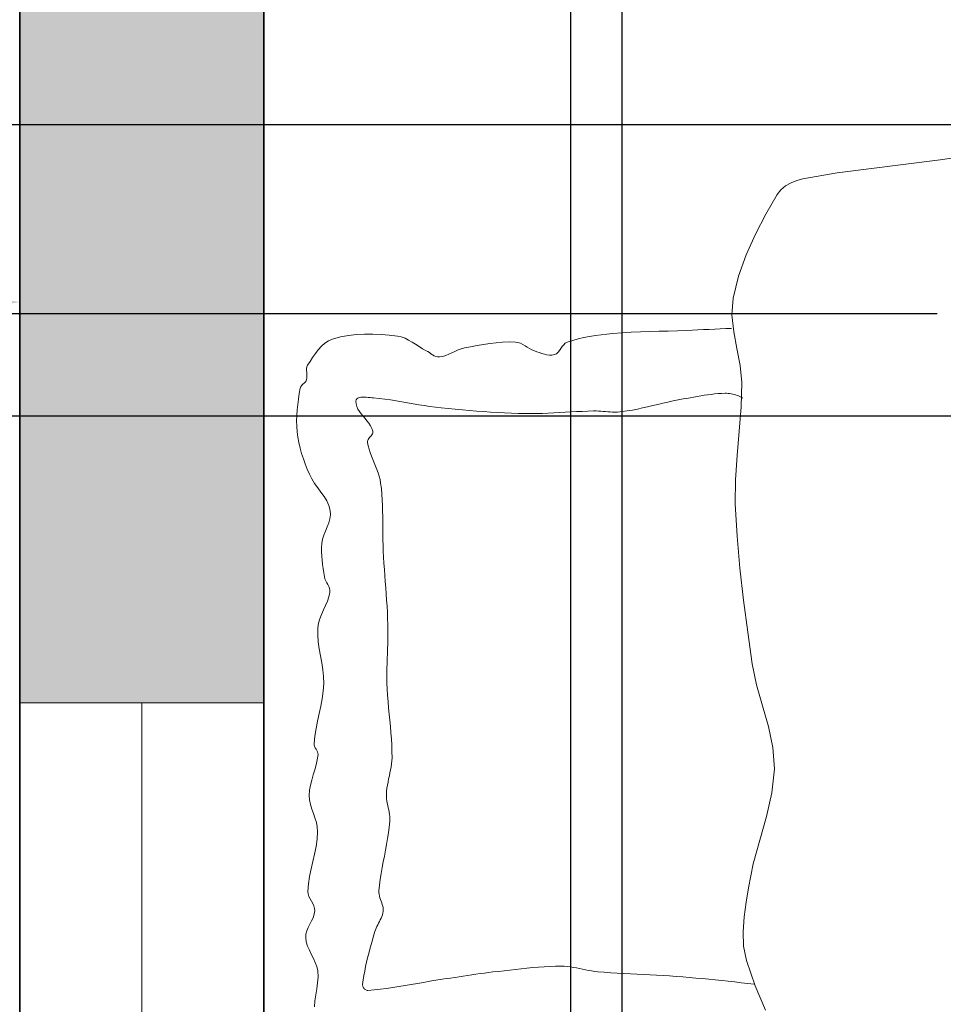
# Model space of a CAD drawing. Units: inches. Extents: x 2656 to 9931, y 1941 to 3068.
# Tile 10 of 46: x 2743 to 2777, y 2533 to 2569. Entities that reach past the tile are written whole.
import ezdxf

# ---------------------------------------------------------------- set-up
doc = ezdxf.new("R2010")
doc.units = ezdxf.units.IN
for name, color, linetype, lineweight in [('A-ANNO-DIMS', 2, 'Continuous', 18), ('A-FURN', 8, 'Continuous', 13), ('A-GLAZ', 4, 'Continuous', 18), ('A-WALL', 7, 'Continuous', 35), ('A-WALL-PATT', 251, 'Continuous', 13)]:
    doc.layers.add(name, color=color, linetype=linetype, lineweight=lineweight)
doc.styles.get("Standard").update_dxf_attribs({"font": 'arial.ttf'})
doc.dimstyles.new('ISO-25', dxfattribs={"dimtxt": 6, "dimasz": 2.5, "dimexe": 1.25, "dimexo": 0.625, "dimtad": 1, "dimdec": 0, "dimlunit": 3, "dimtxsty": 'Standard', "dimcen": 2.5, "dimadec": 0, "dimazin": 0, "dimtfac": 1, "dimtdec": 0, "dimtmove": 0, "dimatfit": 3, "dimfxl": 1, "dimarcsym": 0})

# ---------------------------------------------------------------- blocks, each defined once
blk = doc.blocks.new('*D1')
at = {"layer": 'A-ANNO-DIMS', "color": 0, "lineweight": -2, "transparency": 16777216}
for p, q in [((2728.157, 2559.424), (2728.157, 2560.049)), ((2743.157, 2559.424), (2743.157, 2560.049)), ((2730.657, 2558.799), (2740.657, 2558.799))]:
    blk.add_line(p, q, dxfattribs=at)
at = {"layer": 'A-ANNO-DIMS', "color": 0, "transparency": 16777216}
for points in [[(2730.657, 2559.216), (2730.657, 2558.383), (2728.157, 2558.799)], [(2740.657, 2559.216), (2740.657, 2558.383), (2743.157, 2558.799)]]:
    blk.add_solid(points, dxfattribs=at)
at = {"layer": 'Defpoints', "color": 0, "transparency": 16777216}
for p in [(2728.157, 2558.799), (2743.157, 2558.799), (2743.157, 2558.799)]:
    blk.add_point(p, dxfattribs=at)
at = {"layer": 'A-ANNO-DIMS', "color": 0, "transparency": 16777216, "insert": (2735.657, 2562.49), "char_height": 6, "attachment_point": 5}
blk.add_mtext('1\'3"', dxfattribs=at)
blk = doc.blocks.new('BED-DOUBLE')
for p, q in [((24.929, 61.432), (23.668, 61.237)), ((22.401, 61.078), (21.133, 60.928)), ((23.668, 61.237), (22.401, 61.078)), ((19.868, 60.758), (18.612, 60.54)), ((21.133, 60.928), (19.868, 60.758)), ((17.974, 60.285), (17.799, 60.142)), ((18.176, 60.399), (17.974, 60.285)), ((18.392, 60.483), (18.176, 60.399)), ((18.612, 60.54), (18.392, 60.483)), ((17.664, 59.967), (17.251, 59.242)), ((17.799, 60.142), (17.664, 59.967)), ((17.251, 59.242), (16.864, 58.499)), ((16.864, 58.499), (16.52, 57.736)), ((16.52, 57.736), (16.239, 56.953)), ((16.239, 56.953), (16.039, 56.149)), ((16.039, 56.149), (15.997, 55.53)), ((15.997, 55.53), (16.064, 54.908)), ((2.165, 54.807), (1.867, 54.773)), ((2.466, 54.823), (2.165, 54.807)), ((2.769, 54.822), (2.466, 54.823)), ((3.071, 54.807), (2.769, 54.822)), ((3.373, 54.782), (3.071, 54.807)), ((11.392, 54.817), (11.179, 54.792)), ((11.605, 54.838), (11.392, 54.817)), ((11.945, 54.867), (11.605, 54.838)), ((12.285, 54.889), (11.945, 54.867)), ((12.626, 54.904), (12.285, 54.889)), ((12.968, 54.916), (12.626, 54.904)), ((13.309, 54.925), (12.968, 54.916)), ((13.651, 54.933), (13.309, 54.925)), ((13.992, 54.943), (13.651, 54.933)), ((14.333, 54.956), (13.992, 54.943)), ((14.539, 54.965), (14.333, 54.956)), ((14.745, 54.974), (14.539, 54.965)), ((14.951, 54.984), (14.745, 54.974)), ((15.157, 54.993), (14.951, 54.984)), ((15.363, 55.002), (15.157, 54.993)), ((15.569, 55.012), (15.363, 55.002)), ((15.775, 55.021), (15.569, 55.012)), ((15.98, 55.031), (15.775, 55.021)), ((16.064, 54.908), (16.183, 54.283)), ((0.997, 54.482), (0.871, 54.371)), ((1.134, 54.573), (0.997, 54.482)), ((1.286, 54.638), (1.134, 54.573)), ((1.573, 54.718), (1.286, 54.638)), ((1.867, 54.773), (1.573, 54.718)), ((3.671, 54.748), (3.373, 54.782)), ((3.815, 54.718), (3.671, 54.748)), ((3.953, 54.668), (3.815, 54.718)), ((4.086, 54.602), (3.953, 54.668)), ((4.216, 54.525), (4.086, 54.602)), ((4.344, 54.443), (4.216, 54.525)), ((4.471, 54.359), (4.344, 54.443)), ((6.84, 54.439), (6.605, 54.399)), ((7.076, 54.474), (6.84, 54.439)), ((7.312, 54.503), (7.076, 54.474)), ((7.548, 54.522), (7.312, 54.503)), ((7.785, 54.531), (7.548, 54.522)), ((8.022, 54.528), (7.785, 54.531)), ((8.115, 54.514), (8.022, 54.528)), ((8.204, 54.483), (8.115, 54.514)), ((8.29, 54.44), (8.204, 54.483)), ((8.374, 54.39), (8.29, 54.44)), ((9.858, 54.484), (9.799, 54.428)), ((9.929, 54.522), (9.858, 54.484)), ((10.131, 54.589), (9.929, 54.522)), ((10.337, 54.645), (10.131, 54.589)), ((10.545, 54.692), (10.337, 54.645)), ((10.755, 54.732), (10.545, 54.692)), ((10.967, 54.765), (10.755, 54.732)), ((11.179, 54.792), (10.967, 54.765)), ((0.65, 54.106), (0.55, 53.961)), ((0.756, 54.244), (0.65, 54.106)), ((0.871, 54.371), (0.756, 54.244)), ((4.6, 54.279), (4.471, 54.359)), ((4.732, 54.207), (4.6, 54.279)), ((4.791, 54.174), (4.732, 54.207)), ((4.85, 54.136), (4.791, 54.174)), ((4.909, 54.096), (4.85, 54.136)), ((4.968, 54.058), (4.909, 54.096)), ((5.568, 54.077), (5.454, 54.031)), ((5.68, 54.13), (5.568, 54.077)), ((5.792, 54.184), (5.68, 54.13)), ((5.905, 54.235), (5.792, 54.184)), ((6.02, 54.279), (5.905, 54.235)), ((6.138, 54.31), (6.02, 54.279)), ((6.371, 54.355), (6.138, 54.31)), ((6.605, 54.399), (6.371, 54.355)), ((8.458, 54.336), (8.374, 54.39)), ((8.542, 54.284), (8.458, 54.336)), ((8.628, 54.237), (8.542, 54.284)), ((8.717, 54.201), (8.628, 54.237)), ((8.808, 54.17), (8.717, 54.201)), ((8.9, 54.138), (8.808, 54.17)), ((8.993, 54.107), (8.9, 54.138)), ((9.087, 54.08), (8.993, 54.107)), ((9.181, 54.059), (9.087, 54.08)), ((9.532, 54.097), (9.459, 54.064)), ((9.593, 54.149), (9.532, 54.097)), ((9.647, 54.214), (9.593, 54.149)), ((9.696, 54.287), (9.647, 54.214)), ((9.746, 54.36), (9.696, 54.287)), ((9.799, 54.428), (9.746, 54.36)), ((16.183, 54.283), (16.3, 53.657)), ((0.456, 53.815), (0.365, 53.671)), ((0.55, 53.961), (0.456, 53.815)), ((5.028, 54.024), (4.968, 54.058)), ((5.089, 53.997), (5.028, 54.024)), ((5.153, 53.981), (5.089, 53.997)), ((5.218, 53.978), (5.153, 53.981)), ((5.338, 53.997), (5.218, 53.978)), ((5.454, 54.031), (5.338, 53.997)), ((9.274, 54.048), (9.181, 54.059)), ((9.367, 54.049), (9.274, 54.048)), ((9.459, 54.064), (9.367, 54.049)), ((0.326, 53.548), (0.324, 53.481)), ((0.324, 53.481), (0.33, 53.412)), ((0.337, 53.612), (0.326, 53.548)), ((0.33, 53.412), (0.337, 53.342)), ((0.365, 53.671), (0.337, 53.612)), ((16.3, 53.657), (16.356, 53.03)), ((0.241, 53.017), (0.203, 52.982)), ((0.276, 53.054), (0.241, 53.017)), ((0.306, 53.094), (0.276, 53.054)), ((0.326, 53.138), (0.306, 53.094)), ((0.339, 53.203), (0.326, 53.138)), ((0.337, 53.342), (0.341, 53.272)), ((0.341, 53.272), (0.339, 53.203)), ((16.356, 53.03), (16.332, 52.135)), ((0.058, 52.625), (0.027, 52.426)), ((0.093, 52.823), (0.058, 52.625)), ((0.108, 52.868), (0.093, 52.823)), ((0.134, 52.909), (0.108, 52.868)), ((0.167, 52.946), (0.134, 52.909)), ((0.203, 52.982), (0.167, 52.946)), ((15.359, 52.614), (15.488, 52.625)), ((15.488, 52.625), (15.617, 52.633)), ((15.617, 52.633), (15.747, 52.637)), ((15.747, 52.637), (15.802, 52.637)), ((15.802, 52.637), (15.858, 52.634)), ((15.858, 52.634), (15.913, 52.628)), ((15.913, 52.628), (15.969, 52.619)), ((0.027, 52.426), (0, 52.226)), ((2.14, 52.349), (2.15, 52.398)), ((2.149, 52.246), (2.14, 52.349)), ((2.15, 52.398), (2.175, 52.435)), ((2.175, 52.435), (2.213, 52.463)), ((2.213, 52.463), (2.262, 52.481)), ((2.262, 52.481), (2.32, 52.492)), ((2.32, 52.492), (2.384, 52.497)), ((2.384, 52.497), (2.453, 52.497)), ((2.453, 52.497), (2.525, 52.494)), ((2.525, 52.494), (2.597, 52.487)), ((2.597, 52.487), (2.666, 52.48)), ((2.666, 52.48), (2.731, 52.473)), ((2.731, 52.473), (2.79, 52.468)), ((2.79, 52.468), (3, 52.448)), ((3, 52.448), (3.209, 52.423)), ((3.209, 52.423), (3.417, 52.394)), ((3.417, 52.394), (3.625, 52.362)), ((3.625, 52.362), (3.833, 52.327)), ((3.833, 52.327), (4.041, 52.291)), ((4.041, 52.291), (4.248, 52.254)), ((13.267, 52.226), (13.454, 52.269)), ((13.454, 52.269), (13.641, 52.312)), ((13.641, 52.312), (13.829, 52.354)), ((13.829, 52.354), (14.017, 52.392)), ((14.017, 52.392), (14.206, 52.428)), ((14.206, 52.428), (14.333, 52.451)), ((14.333, 52.451), (14.461, 52.474)), ((14.461, 52.474), (14.589, 52.498)), ((14.589, 52.498), (14.717, 52.521)), ((14.717, 52.521), (14.845, 52.543)), ((14.845, 52.543), (14.973, 52.563)), ((14.973, 52.563), (15.102, 52.582)), ((15.102, 52.582), (15.23, 52.599)), ((15.23, 52.599), (15.359, 52.614)), ((15.969, 52.619), (16.024, 52.608)), ((16.024, 52.608), (16.079, 52.595)), ((16.079, 52.595), (16.133, 52.579)), ((16.133, 52.579), (16.186, 52.561)), ((16.186, 52.561), (16.238, 52.54)), ((16.238, 52.54), (16.289, 52.517)), ((16.289, 52.517), (16.338, 52.491)), ((16.338, 52.491), (16.386, 52.464)), ((-0.022, 52.025), (-0.036, 51.824)), ((0, 52.226), (-0.022, 52.025)), ((2.176, 52.149), (2.149, 52.246)), ((2.219, 52.056), (2.176, 52.149)), ((2.274, 51.966), (2.219, 52.056)), ((2.338, 51.878), (2.274, 51.966)), ((4.248, 52.254), (4.456, 52.218)), ((4.456, 52.218), (4.664, 52.184)), ((4.664, 52.184), (4.872, 52.152)), ((4.872, 52.152), (5.081, 52.123)), ((5.081, 52.123), (5.29, 52.099)), ((5.29, 52.099), (5.548, 52.073)), ((5.548, 52.073), (5.806, 52.048)), ((5.806, 52.048), (6.065, 52.025)), ((6.065, 52.025), (6.323, 52.003)), ((6.323, 52.003), (6.582, 51.982)), ((6.582, 51.982), (6.841, 51.963)), ((6.841, 51.963), (7.1, 51.946)), ((7.1, 51.946), (7.359, 51.931)), ((7.359, 51.931), (7.618, 51.918)), ((7.618, 51.918), (7.877, 51.907)), ((7.877, 51.907), (8.136, 51.898)), ((8.136, 51.898), (8.396, 51.891)), ((8.813, 51.891), (9.022, 51.897)), ((9.022, 51.897), (9.231, 51.905)), ((9.231, 51.905), (9.44, 51.915)), ((9.44, 51.915), (9.648, 51.927)), ((9.648, 51.927), (9.857, 51.939)), ((9.857, 51.939), (10.066, 51.951)), ((10.066, 51.951), (10.275, 51.963)), ((10.275, 51.963), (10.483, 51.973)), ((10.483, 51.973), (10.692, 51.981)), ((10.692, 51.981), (10.901, 51.987)), ((10.901, 51.987), (10.989, 51.987)), ((10.989, 51.987), (11.076, 51.984)), ((11.076, 51.984), (11.164, 51.979)), ((11.164, 51.979), (11.251, 51.973)), ((11.251, 51.973), (11.339, 51.966)), ((11.339, 51.966), (11.427, 51.959)), ((11.427, 51.959), (11.514, 51.953)), ((11.514, 51.953), (11.601, 51.948)), ((11.601, 51.948), (11.689, 51.946)), ((11.689, 51.946), (11.776, 51.947)), ((11.776, 51.947), (11.863, 51.952)), ((11.863, 51.952), (11.95, 51.961)), ((11.95, 51.961), (12.14, 51.989)), ((12.14, 51.989), (12.329, 52.021)), ((12.329, 52.021), (12.517, 52.058)), ((12.517, 52.058), (12.705, 52.097)), ((12.705, 52.097), (12.892, 52.139)), ((12.892, 52.139), (13.08, 52.182)), ((13.08, 52.182), (13.267, 52.226)), ((16.332, 52.135), (16.264, 51.241)), ((-0.036, 51.824), (-0.042, 51.623)), ((-0.042, 51.623), (-0.038, 51.422)), ((2.408, 51.792), (2.338, 51.878)), ((2.481, 51.706), (2.408, 51.792)), ((2.552, 51.62), (2.481, 51.706)), ((2.62, 51.532), (2.552, 51.62)), ((8.396, 51.891), (8.604, 51.889)), ((8.604, 51.889), (8.813, 51.891)), ((-0.038, 51.422), (-0.022, 51.223)), ((-0.022, 51.223), (0.005, 51.02)), ((2.681, 51.441), (2.62, 51.532)), ((2.731, 51.346), (2.681, 51.441)), ((2.768, 51.248), (2.731, 51.346)), ((2.752, 51.141), (2.767, 51.176)), ((2.767, 51.176), (2.773, 51.211)), ((2.773, 51.211), (2.768, 51.248)), ((16.264, 51.241), (16.184, 50.347)), ((0.005, 51.02), (0.042, 50.82)), ((0.042, 50.82), (0.09, 50.62)), ((2.572, 50.868), (2.582, 50.904)), ((2.572, 50.83), (2.572, 50.868)), ((2.597, 50.702), (2.572, 50.83)), ((2.582, 50.904), (2.599, 50.939)), ((2.599, 50.939), (2.622, 50.973)), ((2.622, 50.973), (2.649, 51.007)), ((2.649, 51.007), (2.678, 51.041)), ((2.678, 51.041), (2.706, 51.074)), ((2.706, 51.074), (2.731, 51.108)), ((2.731, 51.108), (2.752, 51.141)), ((0.09, 50.62), (0.145, 50.423)), ((2.63, 50.575), (2.597, 50.702)), ((2.67, 50.45), (2.63, 50.575)), ((2.715, 50.326), (2.67, 50.45)), ((0.145, 50.423), (0.208, 50.227)), ((0.208, 50.227), (0.277, 50.034)), ((2.764, 50.203), (2.715, 50.326)), ((2.815, 50.081), (2.764, 50.203)), ((2.865, 49.958), (2.815, 50.081)), ((16.184, 50.347), (16.125, 49.453)), ((0.277, 50.034), (0.35, 49.842)), ((0.35, 49.842), (0.428, 49.653)), ((2.914, 49.835), (2.865, 49.958)), ((2.959, 49.711), (2.914, 49.835)), ((0.428, 49.653), (0.515, 49.48)), ((0.515, 49.48), (0.62, 49.315)), ((2.999, 49.586), (2.959, 49.711)), ((3.032, 49.459), (2.999, 49.586)), ((3.055, 49.331), (3.032, 49.459)), ((16.125, 49.453), (16.121, 48.558)), ((0.62, 49.315), (0.736, 49.155)), ((0.736, 49.155), (0.854, 48.996)), ((0.854, 48.996), (0.968, 48.836)), ((3.082, 49.123), (3.055, 49.331)), ((3.101, 48.916), (3.082, 49.123)), ((0.968, 48.836), (1.068, 48.671)), ((1.068, 48.671), (1.148, 48.498)), ((3.115, 48.707), (3.101, 48.916)), ((3.124, 48.499), (3.115, 48.707)), ((1.148, 48.498), (1.199, 48.315)), ((1.199, 48.315), (1.208, 48.162)), ((3.129, 48.29), (3.124, 48.499)), ((3.132, 48.081), (3.129, 48.29)), ((16.121, 48.558), (16.187, 47.374)), ((1.186, 48.011), (1.142, 47.861)), ((1.208, 48.162), (1.186, 48.011)), ((3.133, 47.871), (3.132, 48.081)), ((1.02, 47.562), (0.96, 47.411)), ((1.083, 47.712), (1.02, 47.562)), ((1.142, 47.861), (1.083, 47.712)), ((3.134, 47.662), (3.133, 47.871)), ((3.135, 47.452), (3.134, 47.662)), ((0.912, 47.259), (0.885, 47.105)), ((0.96, 47.411), (0.912, 47.259)), ((3.137, 47.243), (3.135, 47.452)), ((3.142, 47.034), (3.137, 47.243)), ((16.187, 47.374), (16.29, 46.193)), ((0.885, 47.105), (0.876, 46.95)), ((0.876, 46.95), (0.876, 46.796)), ((3.151, 46.825), (3.142, 47.034)), ((3.163, 46.599), (3.151, 46.825)), ((0.876, 46.796), (0.882, 46.641)), ((0.882, 46.641), (0.895, 46.486)), ((0.895, 46.486), (0.913, 46.331)), ((3.178, 46.373), (3.163, 46.599)), ((0.913, 46.331), (0.935, 46.177)), ((0.935, 46.177), (0.959, 46.023)), ((3.193, 46.147), (3.178, 46.373)), ((3.209, 45.922), (3.193, 46.147)), ((16.29, 46.193), (16.422, 45.014)), ((0.959, 46.023), (0.984, 45.87)), ((0.984, 45.87), (1.003, 45.798)), ((1.003, 45.798), (1.033, 45.727)), ((1.033, 45.727), (1.069, 45.658)), ((3.226, 45.696), (3.209, 45.922)), ((1.069, 45.658), (1.107, 45.59)), ((1.107, 45.59), (1.143, 45.521)), ((1.143, 45.521), (1.17, 45.452)), ((1.17, 45.452), (1.187, 45.381)), ((1.187, 45.381), (1.187, 45.308)), ((3.243, 45.47), (3.226, 45.696)), ((3.259, 45.245), (3.243, 45.47)), ((1.151, 45.139), (1.095, 44.974)), ((1.187, 45.308), (1.151, 45.139)), ((3.275, 45.019), (3.259, 45.245)), ((3.289, 44.793), (3.275, 45.019)), ((16.422, 45.014), (16.577, 43.838)), ((0.951, 44.651), (0.877, 44.491)), ((1.026, 44.812), (0.951, 44.651)), ((1.095, 44.974), (1.026, 44.812)), ((3.302, 44.567), (3.289, 44.793)), ((0.812, 44.328), (0.763, 44.162)), ((0.877, 44.491), (0.812, 44.328)), ((3.312, 44.341), (3.302, 44.567)), ((3.32, 44.115), (3.312, 44.341)), ((0.738, 43.992), (0.735, 43.734)), ((0.763, 44.162), (0.738, 43.992)), ((3.323, 43.936), (3.32, 44.115)), ((3.323, 43.757), (3.323, 43.936)), ((0.735, 43.734), (0.756, 43.477)), ((3.315, 43.399), (3.32, 43.578)), ((3.32, 43.578), (3.323, 43.757)), ((16.577, 43.838), (16.745, 42.664)), ((0.756, 43.477), (0.793, 43.221)), ((0.793, 43.221), (0.839, 42.964)), ((3.302, 43.041), (3.309, 43.22)), ((3.309, 43.22), (3.315, 43.399)), ((0.839, 42.964), (0.887, 42.708)), ((3.289, 42.683), (3.295, 42.862)), ((3.295, 42.862), (3.302, 43.041)), ((0.887, 42.708), (0.928, 42.451)), ((3.282, 42.325), (3.285, 42.504)), ((3.285, 42.504), (3.289, 42.683)), ((16.745, 42.664), (16.906, 41.889)), ((0.928, 42.451), (0.954, 42.194)), ((0.954, 42.194), (0.959, 41.936)), ((3.283, 42.146), (3.282, 42.325)), ((3.286, 41.967), (3.283, 42.146)), ((0.959, 41.936), (0.94, 41.658)), ((3.296, 41.737), (3.286, 41.967)), ((3.311, 41.506), (3.296, 41.737)), ((16.906, 41.889), (17.122, 41.121)), ((0.902, 41.381), (0.851, 41.106)), ((0.94, 41.658), (0.902, 41.381)), ((3.328, 41.276), (3.311, 41.506)), ((0.851, 41.106), (0.794, 40.832)), ((3.349, 41.046), (3.328, 41.276)), ((3.371, 40.816), (3.349, 41.046)), ((17.122, 41.121), (17.339, 40.355)), ((0.794, 40.832), (0.734, 40.557)), ((3.393, 40.587), (3.371, 40.816)), ((0.679, 40.282), (0.633, 40.006)), ((0.734, 40.557), (0.679, 40.282)), ((3.414, 40.357), (3.393, 40.587)), ((3.434, 40.127), (3.414, 40.357)), ((17.339, 40.355), (17.503, 39.584)), ((0.633, 40.006), (0.601, 39.729)), ((3.45, 39.897), (3.434, 40.127)), ((0.601, 39.729), (0.604, 39.676)), ((0.604, 39.676), (0.621, 39.624)), ((0.621, 39.624), (0.646, 39.574)), ((0.646, 39.574), (0.675, 39.524)), ((3.464, 39.667), (3.45, 39.897)), ((3.472, 39.436), (3.464, 39.667)), ((17.503, 39.584), (17.561, 38.802)), ((0.675, 39.524), (0.704, 39.474)), ((0.704, 39.474), (0.729, 39.424)), ((0.748, 39.32), (0.721, 39.13)), ((0.729, 39.424), (0.745, 39.373)), ((0.745, 39.373), (0.748, 39.32)), ((3.469, 39.093), (3.474, 39.206)), ((3.474, 39.206), (3.472, 39.436)), ((0.678, 38.942), (0.626, 38.755)), ((0.721, 39.13), (0.678, 38.942)), ((3.422, 38.756), (3.443, 38.868)), ((3.443, 38.868), (3.459, 38.98)), ((3.459, 38.98), (3.469, 39.093)), ((0.57, 38.57), (0.516, 38.384)), ((0.626, 38.755), (0.57, 38.57)), ((3.35, 38.422), (3.375, 38.533)), ((3.375, 38.533), (3.399, 38.645)), ((3.399, 38.645), (3.422, 38.756)), ((17.561, 38.802), (17.472, 37.913)), ((0.469, 38.197), (0.437, 38.008)), ((0.516, 38.384), (0.469, 38.197)), ((3.287, 38.087), (3.305, 38.199)), ((3.305, 38.199), (3.326, 38.31)), ((3.326, 38.31), (3.35, 38.422)), ((0.437, 38.008), (0.424, 37.818)), ((0.424, 37.818), (0.437, 37.648)), ((3.266, 37.861), (3.273, 37.974)), ((3.267, 37.778), (3.266, 37.861)), ((3.273, 37.695), (3.267, 37.778)), ((3.273, 37.974), (3.287, 38.087)), ((17.472, 37.913), (17.275, 37.038)), ((0.437, 37.648), (0.472, 37.481)), ((0.472, 37.481), (0.522, 37.316)), ((3.285, 37.612), (3.273, 37.695)), ((3.3, 37.529), (3.285, 37.612)), ((3.317, 37.447), (3.3, 37.529)), ((3.335, 37.364), (3.317, 37.447)), ((0.522, 37.316), (0.579, 37.151)), ((0.579, 37.151), (0.636, 36.987)), ((3.353, 37.282), (3.335, 37.364)), ((3.369, 37.199), (3.353, 37.282)), ((3.383, 37.116), (3.369, 37.199)), ((3.392, 37.034), (3.383, 37.116)), ((3.396, 36.951), (3.392, 37.034)), ((17.275, 37.038), (17.026, 36.168)), ((0.636, 36.987), (0.686, 36.822)), ((0.686, 36.822), (0.72, 36.655)), ((0.72, 36.655), (0.731, 36.485)), ((3.373, 36.652), (3.393, 36.868)), ((3.393, 36.868), (3.396, 36.951)), ((0.731, 36.485), (0.714, 36.207)), ((3.312, 36.223), (3.345, 36.437)), ((3.345, 36.437), (3.373, 36.652)), ((0.674, 35.931), (0.62, 35.656)), ((0.714, 36.207), (0.674, 35.931)), ((3.234, 35.796), (3.274, 36.01)), ((3.274, 36.01), (3.312, 36.223)), ((17.026, 36.168), (16.783, 35.296)), ((0.62, 35.656), (0.558, 35.381)), ((3.15, 35.37), (3.192, 35.583)), ((3.192, 35.583), (3.234, 35.796)), ((0.558, 35.381), (0.495, 35.107)), ((3.11, 35.157), (3.15, 35.37)), ((16.783, 35.296), (16.603, 34.415)), ((0.495, 35.107), (0.438, 34.832)), ((3.039, 34.729), (3.072, 34.943)), ((3.072, 34.943), (3.11, 35.157)), ((0.395, 34.556), (0.373, 34.278)), ((0.438, 34.832), (0.395, 34.556)), ((2.992, 34.298), (3.012, 34.514)), ((3.012, 34.514), (3.039, 34.729)), ((0.373, 34.278), (0.382, 34.185)), ((0.382, 34.185), (0.411, 34.095)), ((2.992, 34.235), (2.992, 34.298)), ((2.999, 34.172), (2.992, 34.235)), ((3.012, 34.109), (2.999, 34.172)), ((16.603, 34.415), (16.521, 33.879)), ((0.411, 34.095), (0.454, 34.007)), ((0.454, 34.007), (0.503, 33.92)), ((0.503, 33.92), (0.552, 33.833)), ((0.552, 33.833), (0.594, 33.745)), ((3.03, 34.047), (3.012, 34.109)), ((3.05, 33.984), (3.03, 34.047)), ((3.073, 33.922), (3.05, 33.984)), ((3.095, 33.86), (3.073, 33.922)), ((3.115, 33.798), (3.095, 33.86)), ((3.132, 33.736), (3.115, 33.798)), ((16.521, 33.879), (16.449, 33.336)), ((0.611, 33.435), (0.569, 33.31)), ((0.594, 33.745), (0.623, 33.655)), ((0.631, 33.562), (0.611, 33.435)), ((0.623, 33.655), (0.631, 33.562)), ((3.098, 33.353), (3.121, 33.416)), ((3.121, 33.416), (3.137, 33.48)), ((3.144, 33.673), (3.132, 33.736)), ((3.137, 33.48), (3.148, 33.546)), ((3.15, 33.61), (3.144, 33.673)), ((3.148, 33.546), (3.15, 33.61)), ((0.45, 33.069), (0.389, 32.949)), ((0.513, 33.189), (0.45, 33.069)), ((0.569, 33.31), (0.513, 33.189)), ((2.915, 32.989), (2.946, 33.049)), ((2.946, 33.049), (2.978, 33.11)), ((2.978, 33.11), (3.011, 33.17)), ((3.011, 33.17), (3.042, 33.231)), ((3.042, 33.231), (3.072, 33.292)), ((3.072, 33.292), (3.098, 33.353)), ((16.449, 33.336), (16.409, 32.793)), ((0.303, 32.703), (0.294, 32.575)), ((0.337, 32.827), (0.303, 32.703)), ((0.389, 32.949), (0.337, 32.827)), ((2.794, 32.639), (2.84, 32.8)), ((2.84, 32.8), (2.86, 32.864)), ((2.86, 32.864), (2.886, 32.927)), ((2.886, 32.927), (2.915, 32.989)), ((16.409, 32.793), (16.428, 32.257)), ((0.294, 32.575), (0.317, 32.415)), ((0.317, 32.415), (0.364, 32.261)), ((2.66, 32.156), (2.704, 32.317)), ((2.704, 32.317), (2.749, 32.479)), ((2.749, 32.479), (2.794, 32.639)), ((0.364, 32.261), (0.428, 32.11)), ((0.428, 32.11), (0.501, 31.961)), ((0.501, 31.961), (0.576, 31.812)), ((2.576, 31.832), (2.617, 31.994)), ((2.617, 31.994), (2.66, 32.156)), ((16.428, 32.257), (16.53, 31.734)), ((0.576, 31.812), (0.645, 31.661)), ((0.645, 31.661), (0.701, 31.508)), ((2.5, 31.506), (2.537, 31.669)), ((2.537, 31.669), (2.576, 31.832)), ((16.53, 31.734), (16.849, 30.803)), ((0.701, 31.508), (0.736, 31.349)), ((0.736, 31.349), (0.748, 31.131)), ((2.437, 31.178), (2.467, 31.343)), ((2.467, 31.343), (2.5, 31.506)), ((6.564, 31.229), (6.409, 31.206)), ((6.72, 31.25), (6.564, 31.229)), ((6.876, 31.271), (6.72, 31.25)), ((7.031, 31.291), (6.876, 31.271)), ((7.188, 31.309), (7.031, 31.291)), ((7.397, 31.332), (7.188, 31.309)), ((7.607, 31.357), (7.397, 31.332)), ((7.816, 31.381), (7.607, 31.357)), ((8.026, 31.405), (7.816, 31.381)), ((8.236, 31.429), (8.026, 31.405)), ((8.446, 31.451), (8.236, 31.429)), ((8.656, 31.471), (8.446, 31.451)), ((8.866, 31.488), (8.656, 31.471)), ((9.076, 31.503), (8.866, 31.488)), ((9.286, 31.514), (9.076, 31.503)), ((9.497, 31.522), (9.286, 31.514)), ((9.707, 31.525), (9.497, 31.522)), ((9.821, 31.521), (9.707, 31.525)), ((9.933, 31.512), (9.821, 31.521)), ((10.045, 31.498), (9.933, 31.512)), ((10.157, 31.48), (10.045, 31.498)), ((10.269, 31.459), (10.157, 31.48)), ((10.381, 31.436), (10.269, 31.459)), ((10.492, 31.412), (10.381, 31.436)), ((10.604, 31.389), (10.492, 31.412)), ((10.715, 31.366), (10.604, 31.389)), ((10.827, 31.346), (10.715, 31.366)), ((10.94, 31.329), (10.827, 31.346)), ((11.052, 31.317), (10.94, 31.329)), ((11.293, 31.297), (11.052, 31.317)), ((11.533, 31.28), (11.293, 31.297)), ((11.774, 31.265), (11.533, 31.28)), ((12.015, 31.252), (11.774, 31.265)), ((12.256, 31.24), (12.015, 31.252)), ((12.497, 31.228), (12.256, 31.24)), ((12.738, 31.217), (12.497, 31.228)), ((12.979, 31.206), (12.738, 31.217)), ((0.733, 30.909), (0.701, 30.686)), ((0.748, 31.131), (0.733, 30.909)), ((2.389, 30.848), (2.411, 31.014)), ((2.389, 30.823), (2.389, 30.848)), ((2.411, 31.014), (2.437, 31.178)), ((4.411, 30.887), (4.183, 30.847)), ((4.638, 30.927), (4.411, 30.887)), ((4.866, 30.967), (4.638, 30.927)), ((5.094, 31.005), (4.866, 30.967)), ((5.322, 31.04), (5.094, 31.005)), ((5.477, 31.063), (5.322, 31.04)), ((5.632, 31.087), (5.477, 31.063)), ((5.788, 31.111), (5.632, 31.087)), ((5.943, 31.135), (5.788, 31.111)), ((6.098, 31.159), (5.943, 31.135)), ((6.254, 31.183), (6.098, 31.159)), ((6.409, 31.206), (6.254, 31.183)), ((13.22, 31.194), (12.979, 31.206)), ((13.461, 31.18), (13.22, 31.194)), ((13.702, 31.165), (13.461, 31.18)), ((13.942, 31.147), (13.702, 31.165)), ((14.182, 31.127), (13.942, 31.147)), ((14.422, 31.107), (14.182, 31.127)), ((14.662, 31.085), (14.422, 31.107)), ((14.902, 31.063), (14.662, 31.085)), ((15.142, 31.04), (14.902, 31.063)), ((15.382, 31.016), (15.142, 31.04)), ((15.621, 30.992), (15.382, 31.016)), ((15.861, 30.966), (15.621, 30.992)), ((16.1, 30.94), (15.861, 30.966)), ((16.34, 30.913), (16.1, 30.94)), ((16.579, 30.885), (16.34, 30.913)), ((16.818, 30.856), (16.579, 30.885)), ((0.701, 30.686), (0.665, 30.462)), ((2.393, 30.798), (2.389, 30.823)), ((2.401, 30.772), (2.393, 30.798)), ((2.413, 30.747), (2.401, 30.772)), ((2.428, 30.723), (2.413, 30.747)), ((2.445, 30.7), (2.428, 30.723)), ((2.465, 30.68), (2.445, 30.7)), ((2.487, 30.662), (2.465, 30.68)), ((2.51, 30.647), (2.487, 30.662)), ((2.534, 30.637), (2.51, 30.647)), ((2.559, 30.631), (2.534, 30.637)), ((2.583, 30.63), (2.559, 30.631)), ((2.813, 30.648), (2.583, 30.63)), ((3.042, 30.672), (2.813, 30.648)), ((3.271, 30.7), (3.042, 30.672)), ((3.5, 30.733), (3.271, 30.7)), ((3.728, 30.769), (3.5, 30.733)), ((3.955, 30.807), (3.728, 30.769)), ((4.183, 30.847), (3.955, 30.807)), ((16.849, 30.803), (17.238, 29.898)), ((0.636, 30.241), (0.624, 30.023)), ((0.665, 30.462), (0.636, 30.241))]:
    blk.add_line(p, q)
blk = doc.blocks.new('WIN-60IN-SASH')
for p, q in [((4.457, 60.033), (-0.043, 60.033)), ((4.457, 0.033), (4.457, 60.033))]:
    blk.add_line(p, q)
blk = doc.blocks.new('*D100')
at = {"layer": 'A-ANNO-DIMS', "color": 0, "lineweight": -2, "transparency": 16777216}
for p, q in [((2696.557, 2565.337), (2696.557, 2603.679)), ((2876.032, 2565.337), (2695.307, 2565.337)), ((2696.557, 2557.1), (2696.557, 2562.837)), ((2876.032, 2554.6), (2695.307, 2554.6))]:
    blk.add_line(p, q, dxfattribs=at)
at = {"layer": 'A-ANNO-DIMS', "color": 0, "transparency": 16777216}
for points in [[(2696.141, 2562.837), (2696.974, 2562.837), (2696.557, 2565.337)], [(2696.141, 2557.1), (2696.974, 2557.1), (2696.557, 2554.6)]]:
    blk.add_solid(points, dxfattribs=at)
at = {"layer": 'Defpoints', "color": 0, "transparency": 16777216}
for p in [(2696.557, 2565.337), (2876.657, 2565.337), (2876.657, 2554.6)]:
    blk.add_point(p, dxfattribs=at)
at = {"layer": 'A-ANNO-DIMS', "color": 0, "transparency": 16777216, "insert": (2692.83, 2585.758), "char_height": 6, "attachment_point": 5, "rotation": 90}
blk.add_mtext('0\'-10 1/2"', dxfattribs=at)
blk = doc.blocks.new('*D113')
at = {"layer": 'A-ANNO-DIMS', "color": 0, "lineweight": -2, "transparency": 16777216}
for p, q in [((2752.157, 2300.725), (2752.157, 2674.45)), ((2809.769, 2300.725), (2809.769, 2674.45)), ((2754.657, 2673.2), (2807.269, 2673.2))]:
    blk.add_line(p, q, dxfattribs=at)
at = {"layer": 'A-ANNO-DIMS', "color": 0, "transparency": 16777216}
for points in [[(2754.657, 2673.617), (2754.657, 2672.784), (2752.157, 2673.2)], [(2807.269, 2673.617), (2807.269, 2672.784), (2809.769, 2673.2)]]:
    blk.add_solid(points, dxfattribs=at)
at = {"layer": 'Defpoints', "color": 0, "transparency": 16777216}
for p in [(2809.769, 2673.2), (2752.157, 2300.1), (2809.769, 2300.1)]:
    blk.add_point(p, dxfattribs=at)
at = {"layer": 'A-ANNO-DIMS', "color": 0, "transparency": 16777216, "insert": (2780.963, 2676.928), "char_height": 6, "attachment_point": 5}
blk.add_mtext('4\'-9 1/2"', dxfattribs=at)
blk = doc.blocks.new('*D128')
at = {"layer": 'A-ANNO-DIMS', "color": 0, "lineweight": -2, "transparency": 16777216}
for p, q in [((2751.532, 2601.771), (2695.307, 2601.771)), ((2696.557, 2599.271), (2696.557, 2560.865)), ((2776.962, 2558.365), (2695.307, 2558.365))]:
    blk.add_line(p, q, dxfattribs=at)
at = {"layer": 'A-ANNO-DIMS', "color": 0, "transparency": 16777216}
for points in [[(2696.141, 2599.271), (2696.974, 2599.271), (2696.557, 2601.771)], [(2696.141, 2560.865), (2696.974, 2560.865), (2696.557, 2558.365)]]:
    blk.add_solid(points, dxfattribs=at)
at = {"layer": 'Defpoints', "color": 0, "transparency": 16777216}
for p in [(2752.157, 2601.771), (2696.557, 2558.365), (2777.587, 2558.365)]:
    blk.add_point(p, dxfattribs=at)
at = {"layer": 'A-ANNO-DIMS', "color": 0, "transparency": 16777216, "insert": (2692.828, 2580.068), "char_height": 6, "attachment_point": 5, "rotation": 90}
blk.add_mtext('3\'-7 1/2"', dxfattribs=at)
blk = doc.blocks.new('*D129')
at = {"layer": 'A-ANNO-DIMS', "color": 0, "lineweight": -2, "transparency": 16777216}
for p, q in [((2752.157, 2601.146), (2752.157, 2009.273)), ((2777.587, 2557.74), (2777.587, 2009.273)), ((2754.657, 2010.523), (2775.087, 2010.523)), ((2777.587, 2010.523), (2811.37, 2010.523))]:
    blk.add_line(p, q, dxfattribs=at)
at = {"layer": 'A-ANNO-DIMS', "color": 0, "transparency": 16777216}
for points in [[(2754.657, 2010.939), (2754.657, 2010.106), (2752.157, 2010.523)], [(2775.087, 2010.939), (2775.087, 2010.106), (2777.587, 2010.523)]]:
    blk.add_solid(points, dxfattribs=at)
at = {"layer": 'Defpoints', "color": 0, "transparency": 16777216}
for p in [(2752.157, 2601.771), (2777.587, 2558.365), (2777.587, 2010.523)]:
    blk.add_point(p, dxfattribs=at)
at = {"layer": 'A-ANNO-DIMS', "color": 0, "transparency": 16777216, "insert": (2795.728, 2014.25), "char_height": 6, "attachment_point": 5}
blk.add_mtext('2\'-1 1/2"', dxfattribs=at)
blk = doc.blocks.new('*D132')
at = {"layer": 'A-ANNO-DIMS', "color": 0, "lineweight": -2, "transparency": 16777216}
for p, q in [((2763.467, 2366.557), (2763.467, 2674.45)), ((2805.965, 2366.557), (2805.965, 2674.45)), ((2765.967, 2673.2), (2803.465, 2673.2))]:
    blk.add_line(p, q, dxfattribs=at)
at = {"layer": 'A-ANNO-DIMS', "color": 0, "transparency": 16777216}
for points in [[(2765.967, 2673.617), (2765.967, 2672.784), (2763.467, 2673.2)], [(2803.465, 2673.617), (2803.465, 2672.784), (2805.965, 2673.2)]]:
    blk.add_solid(points, dxfattribs=at)
at = {"layer": 'Defpoints', "color": 0, "transparency": 16777216}
for p in [(2805.965, 2673.2), (2763.467, 2365.932), (2805.965, 2365.932)]:
    blk.add_point(p, dxfattribs=at)
at = {"layer": 'A-ANNO-DIMS', "color": 0, "transparency": 16777216, "insert": (2784.716, 2676.93), "char_height": 6, "attachment_point": 5}
blk.add_mtext('3\'-6 1/2"', dxfattribs=at)
blk = doc.blocks.new('*D134')
at = {"layer": 'A-ANNO-DIMS', "color": 0, "lineweight": -2, "transparency": 16777216}
for p, q in [((2752.157, 2300.725), (2752.157, 2674.45)), ((2763.467, 2347.433), (2763.467, 2674.45)), ((2754.657, 2673.2), (2760.967, 2673.2)), ((2763.467, 2673.2), (2801.809, 2673.2))]:
    blk.add_line(p, q, dxfattribs=at)
at = {"layer": 'A-ANNO-DIMS', "color": 0, "transparency": 16777216}
for points in [[(2754.657, 2673.617), (2754.657, 2672.784), (2752.157, 2673.2)], [(2760.967, 2673.617), (2760.967, 2672.784), (2763.467, 2673.2)]]:
    blk.add_solid(points, dxfattribs=at)
at = {"layer": 'Defpoints', "color": 0, "transparency": 16777216}
for p in [(2763.467, 2673.2), (2763.467, 2346.808), (2752.157, 2300.1)]:
    blk.add_point(p, dxfattribs=at)
at = {"layer": 'A-ANNO-DIMS', "color": 0, "transparency": 16777216, "insert": (2783.888, 2676.928), "char_height": 6, "attachment_point": 5}
blk.add_mtext('0\'-11 1/2"', dxfattribs=at)
blk = doc.blocks.new('*D136')
at = {"layer": 'A-ANNO-DIMS', "color": 0, "lineweight": -2, "transparency": 16777216}
for p, q in [((2765.357, 2375.042), (2765.357, 2674.45)), ((2779.142, 2375.042), (2779.142, 2674.45)), ((2767.857, 2673.2), (2776.642, 2673.2)), ((2779.142, 2673.2), (2798.277, 2673.2))]:
    blk.add_line(p, q, dxfattribs=at)
at = {"layer": 'A-ANNO-DIMS', "color": 0, "transparency": 16777216}
for points in [[(2767.857, 2673.617), (2767.857, 2672.784), (2765.357, 2673.2)], [(2776.642, 2673.617), (2776.642, 2672.784), (2779.142, 2673.2)]]:
    blk.add_solid(points, dxfattribs=at)
at = {"layer": 'Defpoints', "color": 0, "transparency": 16777216}
for p in [(2779.142, 2673.2), (2765.357, 2374.417), (2779.142, 2374.417)]:
    blk.add_point(p, dxfattribs=at)
at = {"layer": 'A-ANNO-DIMS', "color": 0, "transparency": 16777216, "insert": (2789.959, 2676.838), "char_height": 6, "attachment_point": 5}
blk.add_mtext('1\'-2"', dxfattribs=at)

msp = doc.modelspace()

# ---------------------------------------------------------------- hatches: boundary and pattern name
at = {"layer": 'A-WALL-PATT'}
h = msp.add_hatch(color=256, dxfattribs=at)
h.dxf.hatch_style = 1
h.paths.add_polyline_path([(2858.657, 2623.6), (2752.157, 2623.6), (2752.157, 2614.6), (2858.657, 2614.6)])
h.paths.add_polyline_path([(2893.087, 2623.6), (2876.657, 2623.6), (2876.657, 2614.6), (2893.087, 2614.6), (2893.087, 2619.1)])
h.paths.add_polyline_path([(2946.514, 2623.6), (2917.087, 2623.6), (2917.087, 2614.6), (2946.514, 2614.6), (2946.514, 2619.1)])
h.paths.add_polyline_path([(2989.157, 2623.6), (2970.514, 2623.6), (2970.514, 2614.6), (2989.157, 2614.6)])
h.paths.add_polyline_path([(2998.157, 2605.6), (2989.157, 2605.6), (2989.157, 2523.881), (2998.157, 2523.881)])
h.paths.add_polyline_path([(2935.157, 2614.6), (2930.657, 2614.6), (2930.657, 2554.6), (2876.657, 2554.6), (2876.657, 2565.337), (2872.157, 2565.337), (2872.157, 2444.1), (2876.657, 2444.1), (2876.657, 2550.1), (2946.472, 2550.1), (2946.472, 2554.6), (2935.157, 2554.6)])
h.paths.add_polyline_path([(2989.157, 2554.6), (2982.11, 2554.6), (2976.574, 2554.6), (2976.574, 2550.1), (2982.11, 2550.1), (2989.157, 2550.1)])
h.paths.add_polyline_path([(2876.657, 2614.6), (2872.157, 2614.6), (2872.157, 2595.003), (2876.657, 2595.003)], flags=0)
h.paths.add_polyline_path([(2752.157, 2605.6), (2743.157, 2605.6), (2743.157, 2544.033), (2752.157, 2544.033)])
h.paths.add_polyline_path([(2752.157, 2426.1), (2743.157, 2426.1), (2743.157, 2300.1), (2752.157, 2300.1)])
h.paths.add_polyline_path([(2821.134, 2430.6), (2752.157, 2430.6), (2752.157, 2426.1), (2821.134, 2426.1)])
h.paths.add_polyline_path([(2867.657, 2430.6), (2862.876, 2430.6), (2862.876, 2426.1), (2867.657, 2426.1)])
h.paths.add_polyline_path([(2752.157, 2484.033), (2747.657, 2484.033), (2743.157, 2484.033), (2743.157, 2444.1), (2752.157, 2444.1)])
h.paths.add_polyline_path([(2998.157, 2426.1), (2989.157, 2426.1), (2989.157, 2390.1), (2872.157, 2390.1), (2872.157, 2385.6), (2876.657, 2385.6), (2989.157, 2385.6), (2989.157, 2365.037), (2998.157, 2365.037)])
h.paths.add_polyline_path([(2998.157, 2463.881), (2993.657, 2463.881), (2989.157, 2463.881), (2989.157, 2444.1), (2998.157, 2444.1)])
h.paths.add_polyline_path([(2998.157, 2319.88), (2989.157, 2319.88), (2989.157, 2300.1), (2998.157, 2300.1)])
h.paths.add_polyline_path([(2998.157, 2282.1), (2989.157, 2282.1), (2989.157, 2253.6), (2982.058, 2253.6), (2982.058, 2249.1), (2989.157, 2249.1), (2998.157, 2249.1)])
h.paths.add_polyline_path([(2931.542, 2253.6), (2923.796, 2253.6), (2923.796, 2249.1), (2931.542, 2249.1)])
h.paths.add_polyline_path([(2876.657, 2282.1), (2872.157, 2282.1), (2872.157, 2184.6), (2872.157, 2175.6), (2876.657, 2175.6), (2876.657, 2249.1), (2888.323, 2249.1), (2888.323, 2251.35), (2888.323, 2253.6), (2876.657, 2253.6)])
h.paths.add_polyline_path([(2858.657, 2175.6), (2841.419, 2175.6), (2841.419, 2166.6), (2858.657, 2166.6)])
h.paths.add_polyline_path([(2785.058, 2171.1), (2785.058, 2175.6), (2752.157, 2175.6), (2752.157, 2166.6), (2785.058, 2166.6)])
h.paths.add_polyline_path([(2752.157, 2282.1), (2743.157, 2282.1), (2743.157, 2184.6), (2752.157, 2184.6)])
h.paths.add_polyline_path([(2809.769, 2300.1), (2752.157, 2300.1), (2752.157, 2295.6), (2809.769, 2295.6)])
h.paths.add_polyline_path([(2867.657, 2300.1), (2851.877, 2300.1), (2851.877, 2295.6), (2867.657, 2295.6)])

# ---------------------------------------------------------------- linework, layer by layer
at = {"layer": 'A-GLAZ'}
msp.add_line((2743.157, 2544.033), (2752.157, 2544.033), dxfattribs=at)
at = {"layer": 'A-WALL'}
for p, q in [((2743.157, 2623.6), (2743.157, 2166.6)), ((2752.157, 2614.6), (2752.157, 2166.6))]:
    msp.add_line(p, q, dxfattribs=at)

# ---------------------------------------------------------------- block references
at = {"layer": 'A-FURN'}
msp.add_blockref('BED-DOUBLE', (2753.4, 2502.8), dxfattribs=at)
at = {"layer": 'A-GLAZ'}
msp.add_blockref('WIN-60IN-SASH', (2743.2, 2484), dxfattribs=at)

# ---------------------------------------------------------------- dimensions: what is measured, and where the dimension line sits
at = {"layer": 'A-ANNO-DIMS'}
for base, p1, p2, picture, middle in [((2809.769, 2673.2), (2752.157, 2300.1), (2809.769, 2300.1), '*D113', (2780.963, 2676.928)), ((2763.467, 2673.2), (2752.157, 2300.1), (2763.467, 2346.808), '*D134', (2783.888, 2676.928)), ((2805.965, 2673.2), (2763.467, 2365.932), (2805.965, 2365.932), '*D132', (2784.716, 2676.93)), ((2779.142, 2673.2), (2765.357, 2374.417), (2779.142, 2374.417), '*D136', (2789.959, 2676.838)), ((2777.587, 2010.523), (2752.157, 2601.771), (2777.587, 2558.365), '*D129', (2795.728, 2014.25))]:
    dim = msp.add_linear_dim(base=base, p1=p1, p2=p2, dimstyle='ISO-25', override={"dimdec": 1, "dimlfac": 1, "dimrnd": 0, "dimzin": 1, "dimdsep": 46, "dimlunit": 4, "dimfrac": 2}, dxfattribs=at)
    dim.commit()
    dim.dimension.update_dxf_attribs({"geometry": picture, "text_midpoint": middle})
for base, p1, p2, picture, middle in [((2696.557, 2565.337), (2876.657, 2554.6), (2876.657, 2565.337), '*D100', (2692.83, 2585.758)), ((2696.557, 2558.365), (2752.157, 2601.771), (2777.587, 2558.365), '*D128', (2692.828, 2580.068))]:
    dim = msp.add_linear_dim(base=base, p1=p1, p2=p2, angle=90, dimstyle='ISO-25', override={"dimdec": 1, "dimlfac": 1, "dimrnd": 0, "dimzin": 1, "dimdsep": 46, "dimlunit": 4, "dimfrac": 2}, dxfattribs=at)
    dim.commit()
    dim.dimension.update_dxf_attribs({"geometry": picture, "text_midpoint": middle})
dim = msp.add_linear_dim(base=(2743.157, 2558.799), p1=(2728.157, 2558.799), p2=(2743.157, 2558.799), text='1\'3"', dimstyle='ISO-25', override={"dimclrd": 0, "dimclre": 0, "dimclrt": 0}, dxfattribs=at)
dim.commit()
dim.dimension.update_dxf_attribs({"geometry": '*D1', "text_midpoint": (2735.657, 2562.49)})

doc.saveas('drawing.dxf')
